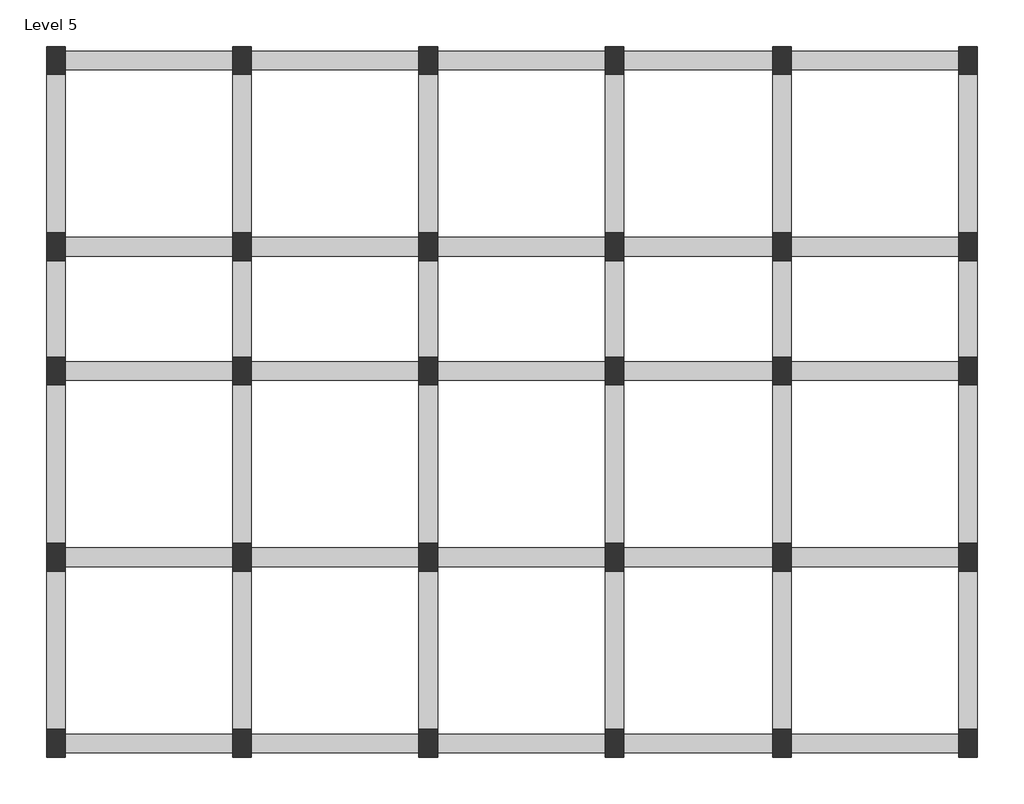
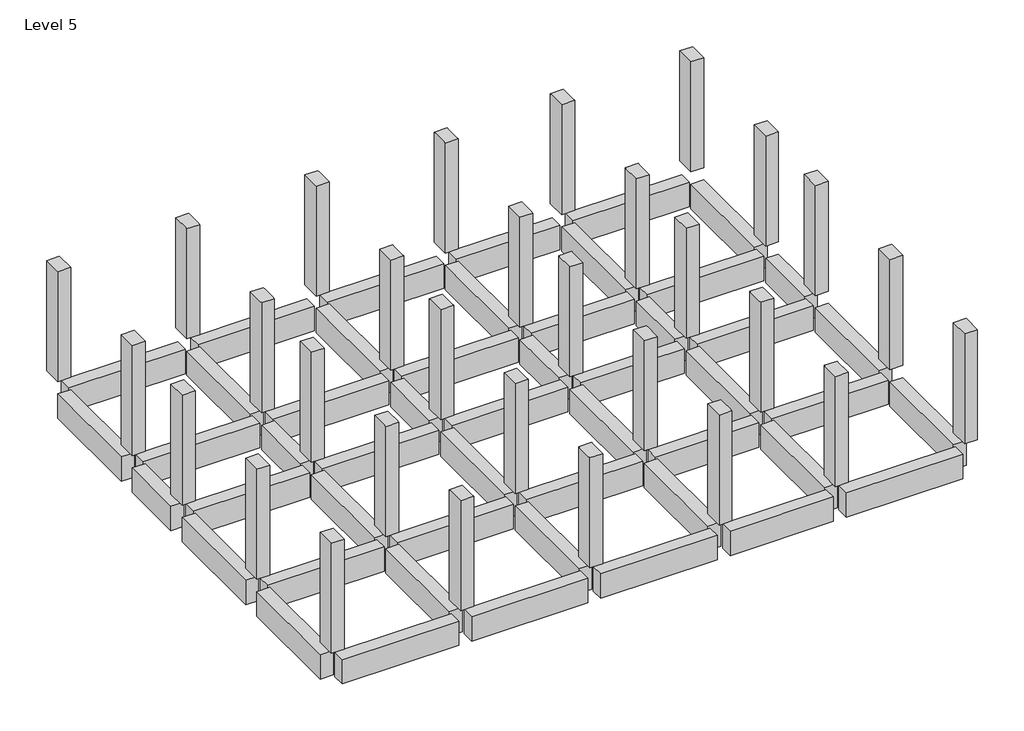
# One storey: 30 columns, 11 beams.
"""IFC4 building model written with IfcOpenShell, lengths in millimetres."""

from ifc_helpers import new_model, si_unit, frame, origin, place, context, project, spatial, polyline, outline, extrude, faceted_brep, element, save

model = new_model("IFC4")

# Units and contexts
model_context = context("Model", 3, world=origin())
ifc_project = project(units=[si_unit("LENGTHUNIT", "METRE", prefix="MILLI")], contexts=[model_context])

# Site, building, storey
site = spatial("IfcSite", under=ifc_project)
building = spatial("IfcBuilding", under=site)
storey = spatial("IfcBuildingStorey", under=building, Name="Level 5", Elevation=12192.0)

# Beams
placement = place(None, origin())
element("IfcBeam", 1, ObjectType="Concrete-Rectangular Beam : 12 x 24", at=placement, inside=storey, context=model_context, shape_type="SweptSolid", body=[
    extrude(outline(polyline([(2607.7603583, 7596.6647757), (2607.7603583, 7291.8647757), (-135.4396417, 7291.8647757), (-135.4396417, 7596.6647757), (2607.7603583, 7596.6647757)])), frame((0.0, 0.0, 11277.6), z_axis=(0.0, 0.0, 1.0), x_axis=(1.0, 0.0, 0.0)), (0.0, 0.0, 1.0), 609.6),
    extrude(outline(polyline([(-12022.6396417, 7291.8647757), (-12022.6396417, 7596.6647757), (-9279.4396417, 7596.6647757), (-9279.4396417, 7291.8647757), (-12022.6396417, 7291.8647757)])), frame((0.0, 0.0, 11277.6), z_axis=(0.0, 0.0, 1.0), x_axis=(1.0, 0.0, 0.0)), (0.0, 0.0, 1.0), 609.6),
    extrude(outline(polyline([(-8974.6396417, 7291.8647757), (-8974.6396417, 7596.6647757), (-6231.4396417, 7596.6647757), (-6231.4396417, 7291.8647757), (-8974.6396417, 7291.8647757)])), frame((0.0, 0.0, 11277.6), z_axis=(0.0, 0.0, 1.0), x_axis=(1.0, 0.0, 0.0)), (0.0, 0.0, 1.0), 609.6),
    extrude(outline(polyline([(-5926.6396417, 7291.8647757), (-5926.6396417, 7596.6647757), (-3183.4396417, 7596.6647757), (-3183.4396417, 7291.8647757), (-5926.6396417, 7291.8647757)])), frame((0.0, 0.0, 11277.6), z_axis=(0.0, 0.0, 1.0), x_axis=(1.0, 0.0, 0.0)), (0.0, 0.0, 1.0), 609.6),
    extrude(outline(polyline([(-2878.6396417, 7291.8647757), (-2878.6396417, 7596.6647757), (-440.2396417, 7596.6647757), (-440.2396417, 7291.8647757), (-2878.6396417, 7291.8647757)])), frame((0.0, 0.0, 11277.6), z_axis=(0.0, 0.0, 1.0), x_axis=(1.0, 0.0, 0.0)), (0.0, 0.0, 1.0), 609.6),
])
element("IfcBeam", 2, ObjectType="Concrete-Rectangular Beam : 12 x 24", at=placement, inside=storey, context=model_context, shape_type="SweptSolid", body=[
    extrude(outline(polyline([(2607.7603583, 10644.6647757), (2607.7603583, 10339.8647757), (-135.4396417, 10339.8647757), (-135.4396417, 10644.6647757), (2607.7603583, 10644.6647757)])), frame((0.0, 0.0, 11277.6), z_axis=(0.0, 0.0, 1.0), x_axis=(1.0, 0.0, 0.0)), (0.0, 0.0, 1.0), 609.6),
    extrude(outline(polyline([(-12022.6396417, 10339.8647757), (-12022.6396417, 10644.6647757), (-9279.4396417, 10644.6647757), (-9279.4396417, 10339.8647757), (-12022.6396417, 10339.8647757)])), frame((0.0, 0.0, 11277.6), z_axis=(0.0, 0.0, 1.0), x_axis=(1.0, 0.0, 0.0)), (0.0, 0.0, 1.0), 609.6),
    extrude(outline(polyline([(-8974.6396417, 10339.8647757), (-8974.6396417, 10644.6647757), (-6231.4396417, 10644.6647757), (-6231.4396417, 10339.8647757), (-8974.6396417, 10339.8647757)])), frame((0.0, 0.0, 11277.6), z_axis=(0.0, 0.0, 1.0), x_axis=(1.0, 0.0, 0.0)), (0.0, 0.0, 1.0), 609.6),
    extrude(outline(polyline([(-5926.6396417, 10339.8647757), (-5926.6396417, 10644.6647757), (-3183.4396417, 10644.6647757), (-3183.4396417, 10339.8647757), (-5926.6396417, 10339.8647757)])), frame((0.0, 0.0, 11277.6), z_axis=(0.0, 0.0, 1.0), x_axis=(1.0, 0.0, 0.0)), (0.0, 0.0, 1.0), 609.6),
    extrude(outline(polyline([(-2878.6396417, 10339.8647757), (-2878.6396417, 10644.6647757), (-440.2396417, 10644.6647757), (-440.2396417, 10339.8647757), (-2878.6396417, 10339.8647757)])), frame((0.0, 0.0, 11277.6), z_axis=(0.0, 0.0, 1.0), x_axis=(1.0, 0.0, 0.0)), (0.0, 0.0, 1.0), 609.6),
])
element("IfcBeam", 3, ObjectType="Concrete-Rectangular Beam : 12 x 24", at=placement, inside=storey, context=model_context, shape_type="SweptSolid", body=[
    extrude(outline(polyline([(2607.7603583, 13692.6647757), (2607.7603583, 13387.8647757), (-135.4396417, 13387.8647757), (-135.4396417, 13692.6647757), (2607.7603583, 13692.6647757)])), frame((0.0, 0.0, 11277.6), z_axis=(0.0, 0.0, 1.0), x_axis=(1.0, 0.0, 0.0)), (0.0, 0.0, 1.0), 609.6),
    extrude(outline(polyline([(-12022.6396417, 13387.8647757), (-12022.6396417, 13692.6647757), (-9279.4396417, 13692.6647757), (-9279.4396417, 13387.8647757), (-12022.6396417, 13387.8647757)])), frame((0.0, 0.0, 11277.6), z_axis=(0.0, 0.0, 1.0), x_axis=(1.0, 0.0, 0.0)), (0.0, 0.0, 1.0), 609.6),
    extrude(outline(polyline([(-8974.6396417, 13387.8647757), (-8974.6396417, 13692.6647757), (-6231.4396417, 13692.6647757), (-6231.4396417, 13387.8647757), (-8974.6396417, 13387.8647757)])), frame((0.0, 0.0, 11277.6), z_axis=(0.0, 0.0, 1.0), x_axis=(1.0, 0.0, 0.0)), (0.0, 0.0, 1.0), 609.6),
    extrude(outline(polyline([(-5926.6396417, 13387.8647757), (-5926.6396417, 13692.6647757), (-3183.4396417, 13692.6647757), (-3183.4396417, 13387.8647757), (-5926.6396417, 13387.8647757)])), frame((0.0, 0.0, 11277.6), z_axis=(0.0, 0.0, 1.0), x_axis=(1.0, 0.0, 0.0)), (0.0, 0.0, 1.0), 609.6),
    extrude(outline(polyline([(-2878.6396417, 13387.8647757), (-2878.6396417, 13692.6647757), (-440.2396417, 13692.6647757), (-440.2396417, 13387.8647757), (-2878.6396417, 13387.8647757)])), frame((0.0, 0.0, 11277.6), z_axis=(0.0, 0.0, 1.0), x_axis=(1.0, 0.0, 0.0)), (0.0, 0.0, 1.0), 609.6),
])
element("IfcBeam", 4, ObjectType="Concrete-Rectangular Beam : 12 x 24", at=placement, inside=storey, context=model_context, shape_type="SweptSolid", body=[
    extrude(outline(polyline([(2607.7603583, 15727.9119241), (2607.7603583, 15423.1119241), (-135.4396417, 15423.1119241), (-135.4396417, 15727.9119241), (2607.7603583, 15727.9119241)])), frame((0.0, 0.0, 11277.6), z_axis=(0.0, 0.0, 1.0), x_axis=(1.0, 0.0, 0.0)), (0.0, 0.0, 1.0), 609.6),
    extrude(outline(polyline([(-12022.6396417, 15423.1119241), (-12022.6396417, 15727.9119241), (-9279.4396417, 15727.9119241), (-9279.4396417, 15423.1119241), (-12022.6396417, 15423.1119241)])), frame((0.0, 0.0, 11277.6), z_axis=(0.0, 0.0, 1.0), x_axis=(1.0, 0.0, 0.0)), (0.0, 0.0, 1.0), 609.6),
    extrude(outline(polyline([(-8974.6396417, 15423.1119241), (-8974.6396417, 15727.9119241), (-6231.4396417, 15727.9119241), (-6231.4396417, 15423.1119241), (-8974.6396417, 15423.1119241)])), frame((0.0, 0.0, 11277.6), z_axis=(0.0, 0.0, 1.0), x_axis=(1.0, 0.0, 0.0)), (0.0, 0.0, 1.0), 609.6),
    extrude(outline(polyline([(-5926.6396417, 15423.1119241), (-5926.6396417, 15727.9119241), (-3183.4396417, 15727.9119241), (-3183.4396417, 15423.1119241), (-5926.6396417, 15423.1119241)])), frame((0.0, 0.0, 11277.6), z_axis=(0.0, 0.0, 1.0), x_axis=(1.0, 0.0, 0.0)), (0.0, 0.0, 1.0), 609.6),
    extrude(outline(polyline([(-2878.6396417, 15423.1119241), (-2878.6396417, 15727.9119241), (-440.2396417, 15727.9119241), (-440.2396417, 15423.1119241), (-2878.6396417, 15423.1119241)])), frame((0.0, 0.0, 11277.6), z_axis=(0.0, 0.0, 1.0), x_axis=(1.0, 0.0, 0.0)), (0.0, 0.0, 1.0), 609.6),
])
element("IfcBeam", 5, ObjectType="Concrete-Rectangular Beam : 12 x 24", at=placement, inside=storey, context=model_context, shape_type="SweptSolid", body=[
    extrude(outline(polyline([(2607.7603583, 18775.9119241), (2607.7603583, 18471.1119241), (-135.4396417, 18471.1119241), (-135.4396417, 18775.9119241), (2607.7603583, 18775.9119241)])), frame((0.0, 0.0, 11277.6), z_axis=(0.0, 0.0, 1.0), x_axis=(1.0, 0.0, 0.0)), (0.0, 0.0, 1.0), 609.6),
    extrude(outline(polyline([(-12022.6396417, 18471.1119241), (-12022.6396417, 18775.9119241), (-9279.4396417, 18775.9119241), (-9279.4396417, 18471.1119241), (-12022.6396417, 18471.1119241)])), frame((0.0, 0.0, 11277.6), z_axis=(0.0, 0.0, 1.0), x_axis=(1.0, 0.0, 0.0)), (0.0, 0.0, 1.0), 609.6),
    extrude(outline(polyline([(-8974.6396417, 18471.1119241), (-8974.6396417, 18775.9119241), (-6231.4396417, 18775.9119241), (-6231.4396417, 18471.1119241), (-8974.6396417, 18471.1119241)])), frame((0.0, 0.0, 11277.6), z_axis=(0.0, 0.0, 1.0), x_axis=(1.0, 0.0, 0.0)), (0.0, 0.0, 1.0), 609.6),
    extrude(outline(polyline([(-5926.6396417, 18471.1119241), (-5926.6396417, 18775.9119241), (-3183.4396417, 18775.9119241), (-3183.4396417, 18471.1119241), (-5926.6396417, 18471.1119241)])), frame((0.0, 0.0, 11277.6), z_axis=(0.0, 0.0, 1.0), x_axis=(1.0, 0.0, 0.0)), (0.0, 0.0, 1.0), 609.6),
    extrude(outline(polyline([(-2878.6396417, 18471.1119241), (-2878.6396417, 18775.9119241), (-440.2396417, 18775.9119241), (-440.2396417, 18471.1119241), (-2878.6396417, 18471.1119241)])), frame((0.0, 0.0, 11277.6), z_axis=(0.0, 0.0, 1.0), x_axis=(1.0, 0.0, 0.0)), (0.0, 0.0, 1.0), 609.6),
])
element("IfcBeam", 6, ObjectType="Concrete-Rectangular Beam : 12 x 24", at=placement, inside=storey, context=model_context, shape_type="SweptSolid", body=[
    extrude(outline(polyline([(-12022.6396417, 7672.8647757), (-12327.4396417, 7672.8647757), (-12327.4396417, 10263.6647757), (-12022.6396417, 10263.6647757), (-12022.6396417, 7672.8647757)])), frame((0.0, 0.0, 11277.6), z_axis=(0.0, 0.0, 1.0), x_axis=(1.0, 0.0, 0.0)), (0.0, 0.0, 1.0), 609.6),
    extrude(outline(polyline([(-12327.4396417, 18394.9119241), (-12022.6396417, 18394.9119241), (-12022.6396417, 15804.1119241), (-12327.4396417, 15804.1119241), (-12327.4396417, 18394.9119241)])), frame((0.0, 0.0, 11277.6), z_axis=(0.0, 0.0, 1.0), x_axis=(1.0, 0.0, 0.0)), (0.0, 0.0, 1.0), 609.6),
    extrude(outline(polyline([(-12022.6396417, 10720.8647757), (-12327.4396417, 10720.8647757), (-12327.4396417, 13311.6647757), (-12022.6396417, 13311.6647757), (-12022.6396417, 10720.8647757)])), frame((0.0, 0.0, 11277.6), z_axis=(0.0, 0.0, 1.0), x_axis=(1.0, 0.0, 0.0)), (0.0, 0.0, 1.0), 609.6),
    extrude(outline(polyline([(-12022.6396417, 13768.8647757), (-12327.4396417, 13768.8647757), (-12327.4396417, 15346.9119241), (-12022.6396417, 15346.9119241), (-12022.6396417, 13768.8647757)])), frame((0.0, 0.0, 11277.6), z_axis=(0.0, 0.0, 1.0), x_axis=(1.0, 0.0, 0.0)), (0.0, 0.0, 1.0), 609.6),
])
element("IfcBeam", 7, ObjectType="Concrete-Rectangular Beam : 12 x 24", at=placement, inside=storey, context=model_context, shape_type="SweptSolid", body=[
    extrude(outline(polyline([(-8974.6396417, 7672.8647757), (-9279.4396417, 7672.8647757), (-9279.4396417, 10263.6647757), (-8974.6396417, 10263.6647757), (-8974.6396417, 7672.8647757)])), frame((0.0, 0.0, 11277.6), z_axis=(0.0, 0.0, 1.0), x_axis=(1.0, 0.0, 0.0)), (0.0, 0.0, 1.0), 609.6),
    extrude(outline(polyline([(-9279.4396417, 18394.9119241), (-8974.6396417, 18394.9119241), (-8974.6396417, 15804.1119241), (-9279.4396417, 15804.1119241), (-9279.4396417, 18394.9119241)])), frame((0.0, 0.0, 11277.6), z_axis=(0.0, 0.0, 1.0), x_axis=(1.0, 0.0, 0.0)), (0.0, 0.0, 1.0), 609.6),
    extrude(outline(polyline([(-8974.6396417, 10720.8647757), (-9279.4396417, 10720.8647757), (-9279.4396417, 13311.6647757), (-8974.6396417, 13311.6647757), (-8974.6396417, 10720.8647757)])), frame((0.0, 0.0, 11277.6), z_axis=(0.0, 0.0, 1.0), x_axis=(1.0, 0.0, 0.0)), (0.0, 0.0, 1.0), 609.6),
    extrude(outline(polyline([(-8974.6396417, 13768.8647757), (-9279.4396417, 13768.8647757), (-9279.4396417, 15346.9119241), (-8974.6396417, 15346.9119241), (-8974.6396417, 13768.8647757)])), frame((0.0, 0.0, 11277.6), z_axis=(0.0, 0.0, 1.0), x_axis=(1.0, 0.0, 0.0)), (0.0, 0.0, 1.0), 609.6),
])
element("IfcBeam", 8, ObjectType="Concrete-Rectangular Beam : 12 x 24", at=placement, inside=storey, context=model_context, shape_type="SweptSolid", body=[
    extrude(outline(polyline([(-5926.6396417, 7672.8647757), (-6231.4396417, 7672.8647757), (-6231.4396417, 10263.6647757), (-5926.6396417, 10263.6647757), (-5926.6396417, 7672.8647757)])), frame((0.0, 0.0, 11277.6), z_axis=(0.0, 0.0, 1.0), x_axis=(1.0, 0.0, 0.0)), (0.0, 0.0, 1.0), 609.6),
    extrude(outline(polyline([(-6231.4396417, 18394.9119241), (-5926.6396417, 18394.9119241), (-5926.6396417, 15804.1119241), (-6231.4396417, 15804.1119241), (-6231.4396417, 18394.9119241)])), frame((0.0, 0.0, 11277.6), z_axis=(0.0, 0.0, 1.0), x_axis=(1.0, 0.0, 0.0)), (0.0, 0.0, 1.0), 609.6),
    extrude(outline(polyline([(-5926.6396417, 10720.8647757), (-6231.4396417, 10720.8647757), (-6231.4396417, 13311.6647757), (-5926.6396417, 13311.6647757), (-5926.6396417, 10720.8647757)])), frame((0.0, 0.0, 11277.6), z_axis=(0.0, 0.0, 1.0), x_axis=(1.0, 0.0, 0.0)), (0.0, 0.0, 1.0), 609.6),
    extrude(outline(polyline([(-5926.6396417, 13768.8647757), (-6231.4396417, 13768.8647757), (-6231.4396417, 15346.9119241), (-5926.6396417, 15346.9119241), (-5926.6396417, 13768.8647757)])), frame((0.0, 0.0, 11277.6), z_axis=(0.0, 0.0, 1.0), x_axis=(1.0, 0.0, 0.0)), (0.0, 0.0, 1.0), 609.6),
])
element("IfcBeam", 9, ObjectType="Concrete-Rectangular Beam : 12 x 24", at=placement, inside=storey, context=model_context, shape_type="SweptSolid", body=[
    extrude(outline(polyline([(-2878.6396417, 7672.8647757), (-3183.4396417, 7672.8647757), (-3183.4396417, 10263.6647757), (-2878.6396417, 10263.6647757), (-2878.6396417, 7672.8647757)])), frame((0.0, 0.0, 11277.6), z_axis=(0.0, 0.0, 1.0), x_axis=(1.0, 0.0, 0.0)), (0.0, 0.0, 1.0), 609.6),
    extrude(outline(polyline([(-3183.4396417, 18394.9119241), (-2878.6396417, 18394.9119241), (-2878.6396417, 15804.1119241), (-3183.4396417, 15804.1119241), (-3183.4396417, 18394.9119241)])), frame((0.0, 0.0, 11277.6), z_axis=(0.0, 0.0, 1.0), x_axis=(1.0, 0.0, 0.0)), (0.0, 0.0, 1.0), 609.6),
    extrude(outline(polyline([(-2878.6396417, 10720.8647757), (-3183.4396417, 10720.8647757), (-3183.4396417, 13311.6647757), (-2878.6396417, 13311.6647757), (-2878.6396417, 10720.8647757)])), frame((0.0, 0.0, 11277.6), z_axis=(0.0, 0.0, 1.0), x_axis=(1.0, 0.0, 0.0)), (0.0, 0.0, 1.0), 609.6),
    extrude(outline(polyline([(-2878.6396417, 13768.8647757), (-3183.4396417, 13768.8647757), (-3183.4396417, 15346.9119241), (-2878.6396417, 15346.9119241), (-2878.6396417, 13768.8647757)])), frame((0.0, 0.0, 11277.6), z_axis=(0.0, 0.0, 1.0), x_axis=(1.0, 0.0, 0.0)), (0.0, 0.0, 1.0), 609.6),
])
element("IfcBeam", 10, ObjectType="Concrete-Rectangular Beam : 12 x 24", at=placement, inside=storey, context=model_context, shape_type="SweptSolid", body=[
    extrude(outline(polyline([(-135.4396417, 7672.8647757), (-440.2396417, 7672.8647757), (-440.2396417, 10263.6647757), (-135.4396417, 10263.6647757), (-135.4396417, 7672.8647757)])), frame((0.0, 0.0, 11277.6), z_axis=(0.0, 0.0, 1.0), x_axis=(1.0, 0.0, 0.0)), (0.0, 0.0, 1.0), 609.6),
    extrude(outline(polyline([(-440.2396417, 18394.9119241), (-135.4396417, 18394.9119241), (-135.4396417, 15804.1119241), (-440.2396417, 15804.1119241), (-440.2396417, 18394.9119241)])), frame((0.0, 0.0, 11277.6), z_axis=(0.0, 0.0, 1.0), x_axis=(1.0, 0.0, 0.0)), (0.0, 0.0, 1.0), 609.6),
    extrude(outline(polyline([(-135.4396417, 10720.8647757), (-440.2396417, 10720.8647757), (-440.2396417, 13311.6647757), (-135.4396417, 13311.6647757), (-135.4396417, 10720.8647757)])), frame((0.0, 0.0, 11277.6), z_axis=(0.0, 0.0, 1.0), x_axis=(1.0, 0.0, 0.0)), (0.0, 0.0, 1.0), 609.6),
    extrude(outline(polyline([(-135.4396417, 13768.8647757), (-440.2396417, 13768.8647757), (-440.2396417, 15346.9119241), (-135.4396417, 15346.9119241), (-135.4396417, 13768.8647757)])), frame((0.0, 0.0, 11277.6), z_axis=(0.0, 0.0, 1.0), x_axis=(1.0, 0.0, 0.0)), (0.0, 0.0, 1.0), 609.6),
])
element("IfcBeam", 11, ObjectType="Concrete-Rectangular Beam : 12 x 24", at=placement, inside=storey, context=model_context, shape_type="SweptSolid", body=[
    extrude(outline(polyline([(2912.5603583, 7672.8647757), (2607.7603583, 7672.8647757), (2607.7603583, 10263.6647757), (2912.5603583, 10263.6647757), (2912.5603583, 7672.8647757)])), frame((0.0, 0.0, 11277.6), z_axis=(0.0, 0.0, 1.0), x_axis=(1.0, 0.0, 0.0)), (0.0, 0.0, 1.0), 609.6),
    extrude(outline(polyline([(2607.7603583, 18394.9119241), (2912.5603583, 18394.9119241), (2912.5603583, 15804.1119241), (2607.7603583, 15804.1119241), (2607.7603583, 18394.9119241)])), frame((0.0, 0.0, 11277.6), z_axis=(0.0, 0.0, 1.0), x_axis=(1.0, 0.0, 0.0)), (0.0, 0.0, 1.0), 609.6),
    extrude(outline(polyline([(2912.5603583, 10720.8647757), (2607.7603583, 10720.8647757), (2607.7603583, 13311.6647757), (2912.5603583, 13311.6647757), (2912.5603583, 10720.8647757)])), frame((0.0, 0.0, 11277.6), z_axis=(0.0, 0.0, 1.0), x_axis=(1.0, 0.0, 0.0)), (0.0, 0.0, 1.0), 609.6),
    extrude(outline(polyline([(2912.5603583, 13768.8647757), (2607.7603583, 13768.8647757), (2607.7603583, 15346.9119241), (2912.5603583, 15346.9119241), (2912.5603583, 13768.8647757)])), frame((0.0, 0.0, 11277.6), z_axis=(0.0, 0.0, 1.0), x_axis=(1.0, 0.0, 0.0)), (0.0, 0.0, 1.0), 609.6),
])

# Columns
element("IfcColumn", 12, ObjectType="Concrete-Rectangular-Column : c1", at=placement, inside=storey, context=model_context, shape_type="SweptSolid", body=[
    extrude(outline(polyline([(-12327.4396417, 7215.6647757), (-12327.4396417, 7672.8647757), (-12022.6396417, 7672.8647757), (-12022.6396417, 7215.6647757), (-12327.4396417, 7215.6647757)])), frame((0.0, 0.0, 12192.0), z_axis=(0.0, 0.0, 1.0), x_axis=(1.0, 0.0, 0.0)), (0.0, 0.0, 1.0), 2743.2),
])
element("IfcColumn", 13, ObjectType="Concrete-Rectangular-Column : c1", at=placement, inside=storey, context=model_context, shape_type="Brep", body=[
    faceted_brep([(-9279.4396417, 7215.6647757, 12192.0), (-9279.4396417, 7672.8647757, 12192.0), (-8974.6396417, 7672.8647757, 12192.0), (-8974.6396417, 7215.6647757, 12192.0), (-9279.4396417, 7215.6647757, 14935.2), (-9279.4396417, 7291.8647757, 14935.2), (-9279.4396417, 7596.6647757, 14935.2), (-9279.4396417, 7672.8647757, 14935.2), (-8974.6396417, 7672.8647757, 14935.2), (-8974.6396417, 7596.6647757, 14935.2), (-8974.6396417, 7291.8647757, 14935.2), (-8974.6396417, 7215.6647757, 14935.2)], [[[0, 1, 2, 3]], [[4, 5, 6, 7, 1, 0]], [[7, 8, 2, 1]], [[8, 9, 10, 11, 3, 2]], [[11, 4, 0, 3]], [[4, 11, 10, 9, 8, 7, 6, 5]]]),
])
element("IfcColumn", 14, ObjectType="Concrete-Rectangular-Column : c1", at=placement, inside=storey, context=model_context, shape_type="Brep", body=[
    faceted_brep([(-6231.4396417, 7215.6647757, 12192.0), (-6231.4396417, 7672.8647757, 12192.0), (-5926.6396417, 7672.8647757, 12192.0), (-5926.6396417, 7215.6647757, 12192.0), (-6231.4396417, 7215.6647757, 14935.2), (-6231.4396417, 7291.8647757, 14935.2), (-6231.4396417, 7596.6647757, 14935.2), (-6231.4396417, 7672.8647757, 14935.2), (-5926.6396417, 7672.8647757, 14935.2), (-5926.6396417, 7596.6647757, 14935.2), (-5926.6396417, 7291.8647757, 14935.2), (-5926.6396417, 7215.6647757, 14935.2)], [[[0, 1, 2, 3]], [[4, 5, 6, 7, 1, 0]], [[7, 8, 2, 1]], [[8, 9, 10, 11, 3, 2]], [[11, 4, 0, 3]], [[4, 11, 10, 9, 8, 7, 6, 5]]]),
])
element("IfcColumn", 15, ObjectType="Concrete-Rectangular-Column : c1", at=placement, inside=storey, context=model_context, shape_type="Brep", body=[
    faceted_brep([(-3183.4396417, 7215.6647757, 12192.0), (-3183.4396417, 7672.8647757, 12192.0), (-2878.6396417, 7672.8647757, 12192.0), (-2878.6396417, 7215.6647757, 12192.0), (-3183.4396417, 7215.6647757, 14935.2), (-3183.4396417, 7291.8647757, 14935.2), (-3183.4396417, 7596.6647757, 14935.2), (-3183.4396417, 7672.8647757, 14935.2), (-2878.6396417, 7672.8647757, 14935.2), (-2878.6396417, 7596.6647757, 14935.2), (-2878.6396417, 7291.8647757, 14935.2), (-2878.6396417, 7215.6647757, 14935.2)], [[[0, 1, 2, 3]], [[4, 5, 6, 7, 1, 0]], [[7, 8, 2, 1]], [[8, 9, 10, 11, 3, 2]], [[11, 4, 0, 3]], [[4, 11, 10, 9, 8, 7, 6, 5]]]),
])
element("IfcColumn", 16, ObjectType="Concrete-Rectangular-Column : c1", at=placement, inside=storey, context=model_context, shape_type="Brep", body=[
    faceted_brep([(-440.2396417, 7215.6647757, 12192.0), (-440.2396417, 7672.8647757, 12192.0), (-135.4396417, 7672.8647757, 12192.0), (-135.4396417, 7215.6647757, 12192.0), (-440.2396417, 7215.6647757, 14935.2), (-440.2396417, 7291.8647757, 14935.2), (-440.2396417, 7596.6647757, 14935.2), (-440.2396417, 7672.8647757, 14935.2), (-135.4396417, 7672.8647757, 14935.2), (-135.4396417, 7596.6647757, 14935.2), (-135.4396417, 7291.8647757, 14935.2), (-135.4396417, 7215.6647757, 14935.2)], [[[0, 1, 2, 3]], [[4, 5, 6, 7, 1, 0]], [[7, 8, 2, 1]], [[8, 9, 10, 11, 3, 2]], [[11, 4, 0, 3]], [[4, 11, 10, 9, 8, 7, 6, 5]]]),
])
element("IfcColumn", 17, ObjectType="Concrete-Rectangular-Column : c1", at=placement, inside=storey, context=model_context, shape_type="SweptSolid", body=[
    extrude(outline(polyline([(2607.7603583, 7215.6647757), (2607.7603583, 7672.8647757), (2912.5603583, 7672.8647757), (2912.5603583, 7215.6647757), (2607.7603583, 7215.6647757)])), frame((0.0, 0.0, 12192.0), z_axis=(0.0, 0.0, 1.0), x_axis=(1.0, 0.0, 0.0)), (0.0, 0.0, 1.0), 2743.2),
])
element("IfcColumn", 18, ObjectType="Concrete-Rectangular-Column : c1", at=placement, inside=storey, context=model_context, shape_type="Brep", body=[
    faceted_brep([(-12327.4396417, 10263.6647757, 12192.0), (-12327.4396417, 10720.8647757, 12192.0), (-12022.6396417, 10720.8647757, 12192.0), (-12022.6396417, 10263.6647757, 12192.0), (-12327.4396417, 10263.6647757, 14935.2), (-12327.4396417, 10720.8647757, 14935.2), (-12327.4396417, 10720.8647757, 14325.6), (-12327.4396417, 10263.6647757, 14325.6), (-12022.6396417, 10720.8647757, 14935.2), (-12022.6396417, 10720.8647757, 14325.6), (-12022.6396417, 10263.6647757, 14935.2), (-12022.6396417, 10263.6647757, 14325.6)], [[[0, 1, 2, 3]], [[4, 5, 6, 1, 0, 7]], [[5, 8, 9, 2, 1, 6]], [[8, 10, 11, 3, 2, 9]], [[10, 4, 7, 0, 3, 11]], [[4, 10, 8, 5]]]),
])
element("IfcColumn", 19, ObjectType="Concrete-Rectangular-Column : c1", at=placement, inside=storey, context=model_context, shape_type="Brep", body=[
    faceted_brep([(-9279.4396417, 10263.6647757, 12192.0), (-9279.4396417, 10720.8647757, 12192.0), (-8974.6396417, 10720.8647757, 12192.0), (-8974.6396417, 10263.6647757, 12192.0), (-9279.4396417, 10263.6647757, 14935.2), (-9279.4396417, 10339.8647757, 14935.2), (-9279.4396417, 10644.6647757, 14935.2), (-9279.4396417, 10720.8647757, 14935.2), (-9279.4396417, 10720.8647757, 14325.6), (-9279.4396417, 10263.6647757, 14325.6), (-8974.6396417, 10720.8647757, 14935.2), (-8974.6396417, 10720.8647757, 14325.6), (-8974.6396417, 10644.6647757, 14935.2), (-8974.6396417, 10339.8647757, 14935.2), (-8974.6396417, 10263.6647757, 14935.2), (-8974.6396417, 10263.6647757, 14325.6)], [[[0, 1, 2, 3]], [[4, 5, 6, 7, 8, 1, 0, 9]], [[7, 10, 11, 2, 1, 8]], [[10, 12, 13, 14, 15, 3, 2, 11]], [[14, 4, 9, 0, 3, 15]], [[4, 14, 13, 12, 10, 7, 6, 5]]]),
])
element("IfcColumn", 20, ObjectType="Concrete-Rectangular-Column : c1", at=placement, inside=storey, context=model_context, shape_type="Brep", body=[
    faceted_brep([(-6231.4396417, 10263.6647757, 12192.0), (-6231.4396417, 10720.8647757, 12192.0), (-5926.6396417, 10720.8647757, 12192.0), (-5926.6396417, 10263.6647757, 12192.0), (-6231.4396417, 10263.6647757, 14935.2), (-6231.4396417, 10339.8647757, 14935.2), (-6231.4396417, 10644.6647757, 14935.2), (-6231.4396417, 10720.8647757, 14935.2), (-6231.4396417, 10720.8647757, 14325.6), (-6231.4396417, 10263.6647757, 14325.6), (-5926.6396417, 10720.8647757, 14935.2), (-5926.6396417, 10720.8647757, 14325.6), (-5926.6396417, 10644.6647757, 14935.2), (-5926.6396417, 10339.8647757, 14935.2), (-5926.6396417, 10263.6647757, 14935.2), (-5926.6396417, 10263.6647757, 14325.6)], [[[0, 1, 2, 3]], [[4, 5, 6, 7, 8, 1, 0, 9]], [[7, 10, 11, 2, 1, 8]], [[10, 12, 13, 14, 15, 3, 2, 11]], [[14, 4, 9, 0, 3, 15]], [[4, 14, 13, 12, 10, 7, 6, 5]]]),
])
element("IfcColumn", 21, ObjectType="Concrete-Rectangular-Column : c1", at=placement, inside=storey, context=model_context, shape_type="Brep", body=[
    faceted_brep([(-3183.4396417, 10263.6647757, 12192.0), (-3183.4396417, 10720.8647757, 12192.0), (-2878.6396417, 10720.8647757, 12192.0), (-2878.6396417, 10263.6647757, 12192.0), (-3183.4396417, 10263.6647757, 14935.2), (-3183.4396417, 10339.8647757, 14935.2), (-3183.4396417, 10644.6647757, 14935.2), (-3183.4396417, 10720.8647757, 14935.2), (-3183.4396417, 10720.8647757, 14325.6), (-3183.4396417, 10263.6647757, 14325.6), (-2878.6396417, 10720.8647757, 14935.2), (-2878.6396417, 10720.8647757, 14325.6), (-2878.6396417, 10644.6647757, 14935.2), (-2878.6396417, 10339.8647757, 14935.2), (-2878.6396417, 10263.6647757, 14935.2), (-2878.6396417, 10263.6647757, 14325.6)], [[[0, 1, 2, 3]], [[4, 5, 6, 7, 8, 1, 0, 9]], [[7, 10, 11, 2, 1, 8]], [[10, 12, 13, 14, 15, 3, 2, 11]], [[14, 4, 9, 0, 3, 15]], [[4, 14, 13, 12, 10, 7, 6, 5]]]),
])
element("IfcColumn", 22, ObjectType="Concrete-Rectangular-Column : c1", at=placement, inside=storey, context=model_context, shape_type="Brep", body=[
    faceted_brep([(-440.2396417, 10263.6647757, 12192.0), (-440.2396417, 10720.8647757, 12192.0), (-135.4396417, 10720.8647757, 12192.0), (-135.4396417, 10263.6647757, 12192.0), (-440.2396417, 10263.6647757, 14935.2), (-440.2396417, 10339.8647757, 14935.2), (-440.2396417, 10644.6647757, 14935.2), (-440.2396417, 10720.8647757, 14935.2), (-440.2396417, 10720.8647757, 14325.6), (-440.2396417, 10263.6647757, 14325.6), (-135.4396417, 10720.8647757, 14935.2), (-135.4396417, 10720.8647757, 14325.6), (-135.4396417, 10644.6647757, 14935.2), (-135.4396417, 10339.8647757, 14935.2), (-135.4396417, 10263.6647757, 14935.2), (-135.4396417, 10263.6647757, 14325.6)], [[[0, 1, 2, 3]], [[4, 5, 6, 7, 8, 1, 0, 9]], [[7, 10, 11, 2, 1, 8]], [[10, 12, 13, 14, 15, 3, 2, 11]], [[14, 4, 9, 0, 3, 15]], [[4, 14, 13, 12, 10, 7, 6, 5]]]),
])
element("IfcColumn", 23, ObjectType="Concrete-Rectangular-Column : c1", at=placement, inside=storey, context=model_context, shape_type="Brep", body=[
    faceted_brep([(2607.7603583, 10263.6647757, 12192.0), (2607.7603583, 10720.8647757, 12192.0), (2912.5603583, 10720.8647757, 12192.0), (2912.5603583, 10263.6647757, 12192.0), (2607.7603583, 10263.6647757, 14935.2), (2607.7603583, 10720.8647757, 14935.2), (2607.7603583, 10720.8647757, 14325.6), (2607.7603583, 10263.6647757, 14325.6), (2912.5603583, 10720.8647757, 14935.2), (2912.5603583, 10720.8647757, 14325.6), (2912.5603583, 10263.6647757, 14935.2), (2912.5603583, 10263.6647757, 14325.6)], [[[0, 1, 2, 3]], [[4, 5, 6, 1, 0, 7]], [[5, 8, 9, 2, 1, 6]], [[8, 10, 11, 3, 2, 9]], [[10, 4, 7, 0, 3, 11]], [[4, 10, 8, 5]]]),
])
element("IfcColumn", 24, ObjectType="Concrete-Rectangular-Column : c1", at=placement, inside=storey, context=model_context, shape_type="Brep", body=[
    faceted_brep([(-12327.4396417, 13311.6647757, 12192.0), (-12327.4396417, 13768.8647757, 12192.0), (-12022.6396417, 13768.8647757, 12192.0), (-12022.6396417, 13311.6647757, 12192.0), (-12327.4396417, 13311.6647757, 14935.2), (-12327.4396417, 13768.8647757, 14935.2), (-12327.4396417, 13768.8647757, 14325.6), (-12327.4396417, 13311.6647757, 14325.6), (-12022.6396417, 13768.8647757, 14935.2), (-12022.6396417, 13768.8647757, 14325.6), (-12022.6396417, 13311.6647757, 14935.2), (-12022.6396417, 13311.6647757, 14325.6)], [[[0, 1, 2, 3]], [[4, 5, 6, 1, 0, 7]], [[5, 8, 9, 2, 1, 6]], [[8, 10, 11, 3, 2, 9]], [[10, 4, 7, 0, 3, 11]], [[4, 10, 8, 5]]]),
])
element("IfcColumn", 25, ObjectType="Concrete-Rectangular-Column : c1", at=placement, inside=storey, context=model_context, shape_type="Brep", body=[
    faceted_brep([(-9279.4396417, 13311.6647757, 12192.0), (-9279.4396417, 13768.8647757, 12192.0), (-8974.6396417, 13768.8647757, 12192.0), (-8974.6396417, 13311.6647757, 12192.0), (-9279.4396417, 13311.6647757, 14935.2), (-9279.4396417, 13387.8647757, 14935.2), (-9279.4396417, 13692.6647757, 14935.2), (-9279.4396417, 13768.8647757, 14935.2), (-9279.4396417, 13768.8647757, 14325.6), (-9279.4396417, 13311.6647757, 14325.6), (-8974.6396417, 13768.8647757, 14935.2), (-8974.6396417, 13768.8647757, 14325.6), (-8974.6396417, 13692.6647757, 14935.2), (-8974.6396417, 13387.8647757, 14935.2), (-8974.6396417, 13311.6647757, 14935.2), (-8974.6396417, 13311.6647757, 14325.6)], [[[0, 1, 2, 3]], [[4, 5, 6, 7, 8, 1, 0, 9]], [[7, 10, 11, 2, 1, 8]], [[10, 12, 13, 14, 15, 3, 2, 11]], [[14, 4, 9, 0, 3, 15]], [[4, 14, 13, 12, 10, 7, 6, 5]]]),
])
element("IfcColumn", 26, ObjectType="Concrete-Rectangular-Column : c1", at=placement, inside=storey, context=model_context, shape_type="Brep", body=[
    faceted_brep([(-6231.4396417, 13311.6647757, 12192.0), (-6231.4396417, 13768.8647757, 12192.0), (-5926.6396417, 13768.8647757, 12192.0), (-5926.6396417, 13311.6647757, 12192.0), (-6231.4396417, 13311.6647757, 14935.2), (-6231.4396417, 13387.8647757, 14935.2), (-6231.4396417, 13692.6647757, 14935.2), (-6231.4396417, 13768.8647757, 14935.2), (-6231.4396417, 13768.8647757, 14325.6), (-6231.4396417, 13311.6647757, 14325.6), (-5926.6396417, 13768.8647757, 14935.2), (-5926.6396417, 13768.8647757, 14325.6), (-5926.6396417, 13692.6647757, 14935.2), (-5926.6396417, 13387.8647757, 14935.2), (-5926.6396417, 13311.6647757, 14935.2), (-5926.6396417, 13311.6647757, 14325.6)], [[[0, 1, 2, 3]], [[4, 5, 6, 7, 8, 1, 0, 9]], [[7, 10, 11, 2, 1, 8]], [[10, 12, 13, 14, 15, 3, 2, 11]], [[14, 4, 9, 0, 3, 15]], [[4, 14, 13, 12, 10, 7, 6, 5]]]),
])
element("IfcColumn", 27, ObjectType="Concrete-Rectangular-Column : c1", at=placement, inside=storey, context=model_context, shape_type="Brep", body=[
    faceted_brep([(-3183.4396417, 13311.6647757, 12192.0), (-3183.4396417, 13768.8647757, 12192.0), (-2878.6396417, 13768.8647757, 12192.0), (-2878.6396417, 13311.6647757, 12192.0), (-3183.4396417, 13311.6647757, 14935.2), (-3183.4396417, 13387.8647757, 14935.2), (-3183.4396417, 13692.6647757, 14935.2), (-3183.4396417, 13768.8647757, 14935.2), (-3183.4396417, 13768.8647757, 14325.6), (-3183.4396417, 13311.6647757, 14325.6), (-2878.6396417, 13768.8647757, 14935.2), (-2878.6396417, 13768.8647757, 14325.6), (-2878.6396417, 13692.6647757, 14935.2), (-2878.6396417, 13387.8647757, 14935.2), (-2878.6396417, 13311.6647757, 14935.2), (-2878.6396417, 13311.6647757, 14325.6)], [[[0, 1, 2, 3]], [[4, 5, 6, 7, 8, 1, 0, 9]], [[7, 10, 11, 2, 1, 8]], [[10, 12, 13, 14, 15, 3, 2, 11]], [[14, 4, 9, 0, 3, 15]], [[4, 14, 13, 12, 10, 7, 6, 5]]]),
])
element("IfcColumn", 28, ObjectType="Concrete-Rectangular-Column : c1", at=placement, inside=storey, context=model_context, shape_type="Brep", body=[
    faceted_brep([(-440.2396417, 13311.6647757, 12192.0), (-440.2396417, 13768.8647757, 12192.0), (-135.4396417, 13768.8647757, 12192.0), (-135.4396417, 13311.6647757, 12192.0), (-440.2396417, 13311.6647757, 14935.2), (-440.2396417, 13387.8647757, 14935.2), (-440.2396417, 13692.6647757, 14935.2), (-440.2396417, 13768.8647757, 14935.2), (-440.2396417, 13768.8647757, 14325.6), (-440.2396417, 13311.6647757, 14325.6), (-135.4396417, 13768.8647757, 14935.2), (-135.4396417, 13768.8647757, 14325.6), (-135.4396417, 13692.6647757, 14935.2), (-135.4396417, 13387.8647757, 14935.2), (-135.4396417, 13311.6647757, 14935.2), (-135.4396417, 13311.6647757, 14325.6)], [[[0, 1, 2, 3]], [[4, 5, 6, 7, 8, 1, 0, 9]], [[7, 10, 11, 2, 1, 8]], [[10, 12, 13, 14, 15, 3, 2, 11]], [[14, 4, 9, 0, 3, 15]], [[4, 14, 13, 12, 10, 7, 6, 5]]]),
])
element("IfcColumn", 29, ObjectType="Concrete-Rectangular-Column : c1", at=placement, inside=storey, context=model_context, shape_type="Brep", body=[
    faceted_brep([(2607.7603583, 13311.6647757, 12192.0), (2607.7603583, 13768.8647757, 12192.0), (2912.5603583, 13768.8647757, 12192.0), (2912.5603583, 13311.6647757, 12192.0), (2607.7603583, 13311.6647757, 14935.2), (2607.7603583, 13768.8647757, 14935.2), (2607.7603583, 13768.8647757, 14325.6), (2607.7603583, 13311.6647757, 14325.6), (2912.5603583, 13768.8647757, 14935.2), (2912.5603583, 13768.8647757, 14325.6), (2912.5603583, 13311.6647757, 14935.2), (2912.5603583, 13311.6647757, 14325.6)], [[[0, 1, 2, 3]], [[4, 5, 6, 1, 0, 7]], [[5, 8, 9, 2, 1, 6]], [[8, 10, 11, 3, 2, 9]], [[10, 4, 7, 0, 3, 11]], [[4, 10, 8, 5]]]),
])
element("IfcColumn", 30, ObjectType="Concrete-Rectangular-Column : c1", at=placement, inside=storey, context=model_context, shape_type="Brep", body=[
    faceted_brep([(-12327.4396417, 15346.9119241, 12192.0), (-12327.4396417, 15804.1119241, 12192.0), (-12022.6396417, 15804.1119241, 12192.0), (-12022.6396417, 15346.9119241, 12192.0), (-12327.4396417, 15346.9119241, 14935.2), (-12327.4396417, 15804.1119241, 14935.2), (-12327.4396417, 15804.1119241, 14325.6), (-12327.4396417, 15346.9119241, 14325.6), (-12022.6396417, 15804.1119241, 14935.2), (-12022.6396417, 15804.1119241, 14325.6), (-12022.6396417, 15346.9119241, 14935.2), (-12022.6396417, 15346.9119241, 14325.6)], [[[0, 1, 2, 3]], [[4, 5, 6, 1, 0, 7]], [[5, 8, 9, 2, 1, 6]], [[8, 10, 11, 3, 2, 9]], [[10, 4, 7, 0, 3, 11]], [[4, 10, 8, 5]]]),
])
element("IfcColumn", 31, ObjectType="Concrete-Rectangular-Column : c1", at=placement, inside=storey, context=model_context, shape_type="Brep", body=[
    faceted_brep([(-9279.4396417, 15346.9119241, 12192.0), (-9279.4396417, 15804.1119241, 12192.0), (-8974.6396417, 15804.1119241, 12192.0), (-8974.6396417, 15346.9119241, 12192.0), (-9279.4396417, 15346.9119241, 14935.2), (-9279.4396417, 15423.1119241, 14935.2), (-9279.4396417, 15727.9119241, 14935.2), (-9279.4396417, 15804.1119241, 14935.2), (-9279.4396417, 15804.1119241, 14325.6), (-9279.4396417, 15346.9119241, 14325.6), (-8974.6396417, 15804.1119241, 14935.2), (-8974.6396417, 15804.1119241, 14325.6), (-8974.6396417, 15727.9119241, 14935.2), (-8974.6396417, 15423.1119241, 14935.2), (-8974.6396417, 15346.9119241, 14935.2), (-8974.6396417, 15346.9119241, 14325.6)], [[[0, 1, 2, 3]], [[4, 5, 6, 7, 8, 1, 0, 9]], [[7, 10, 11, 2, 1, 8]], [[10, 12, 13, 14, 15, 3, 2, 11]], [[14, 4, 9, 0, 3, 15]], [[4, 14, 13, 12, 10, 7, 6, 5]]]),
])
element("IfcColumn", 32, ObjectType="Concrete-Rectangular-Column : c1", at=placement, inside=storey, context=model_context, shape_type="Brep", body=[
    faceted_brep([(-6231.4396417, 15346.9119241, 12192.0), (-6231.4396417, 15804.1119241, 12192.0), (-5926.6396417, 15804.1119241, 12192.0), (-5926.6396417, 15346.9119241, 12192.0), (-6231.4396417, 15346.9119241, 14935.2), (-6231.4396417, 15423.1119241, 14935.2), (-6231.4396417, 15727.9119241, 14935.2), (-6231.4396417, 15804.1119241, 14935.2), (-6231.4396417, 15804.1119241, 14325.6), (-6231.4396417, 15346.9119241, 14325.6), (-5926.6396417, 15804.1119241, 14935.2), (-5926.6396417, 15804.1119241, 14325.6), (-5926.6396417, 15727.9119241, 14935.2), (-5926.6396417, 15423.1119241, 14935.2), (-5926.6396417, 15346.9119241, 14935.2), (-5926.6396417, 15346.9119241, 14325.6)], [[[0, 1, 2, 3]], [[4, 5, 6, 7, 8, 1, 0, 9]], [[7, 10, 11, 2, 1, 8]], [[10, 12, 13, 14, 15, 3, 2, 11]], [[14, 4, 9, 0, 3, 15]], [[4, 14, 13, 12, 10, 7, 6, 5]]]),
])
element("IfcColumn", 33, ObjectType="Concrete-Rectangular-Column : c1", at=placement, inside=storey, context=model_context, shape_type="Brep", body=[
    faceted_brep([(-3183.4396417, 15346.9119241, 12192.0), (-3183.4396417, 15804.1119241, 12192.0), (-2878.6396417, 15804.1119241, 12192.0), (-2878.6396417, 15346.9119241, 12192.0), (-3183.4396417, 15346.9119241, 14935.2), (-3183.4396417, 15423.1119241, 14935.2), (-3183.4396417, 15727.9119241, 14935.2), (-3183.4396417, 15804.1119241, 14935.2), (-3183.4396417, 15804.1119241, 14325.6), (-3183.4396417, 15346.9119241, 14325.6), (-2878.6396417, 15804.1119241, 14935.2), (-2878.6396417, 15804.1119241, 14325.6), (-2878.6396417, 15727.9119241, 14935.2), (-2878.6396417, 15423.1119241, 14935.2), (-2878.6396417, 15346.9119241, 14935.2), (-2878.6396417, 15346.9119241, 14325.6)], [[[0, 1, 2, 3]], [[4, 5, 6, 7, 8, 1, 0, 9]], [[7, 10, 11, 2, 1, 8]], [[10, 12, 13, 14, 15, 3, 2, 11]], [[14, 4, 9, 0, 3, 15]], [[4, 14, 13, 12, 10, 7, 6, 5]]]),
])
element("IfcColumn", 34, ObjectType="Concrete-Rectangular-Column : c1", at=placement, inside=storey, context=model_context, shape_type="Brep", body=[
    faceted_brep([(-440.2396417, 15346.9119241, 12192.0), (-440.2396417, 15804.1119241, 12192.0), (-135.4396417, 15804.1119241, 12192.0), (-135.4396417, 15346.9119241, 12192.0), (-440.2396417, 15346.9119241, 14935.2), (-440.2396417, 15423.1119241, 14935.2), (-440.2396417, 15727.9119241, 14935.2), (-440.2396417, 15804.1119241, 14935.2), (-440.2396417, 15804.1119241, 14325.6), (-440.2396417, 15346.9119241, 14325.6), (-135.4396417, 15804.1119241, 14935.2), (-135.4396417, 15804.1119241, 14325.6), (-135.4396417, 15727.9119241, 14935.2), (-135.4396417, 15423.1119241, 14935.2), (-135.4396417, 15346.9119241, 14935.2), (-135.4396417, 15346.9119241, 14325.6)], [[[0, 1, 2, 3]], [[4, 5, 6, 7, 8, 1, 0, 9]], [[7, 10, 11, 2, 1, 8]], [[10, 12, 13, 14, 15, 3, 2, 11]], [[14, 4, 9, 0, 3, 15]], [[4, 14, 13, 12, 10, 7, 6, 5]]]),
])
element("IfcColumn", 35, ObjectType="Concrete-Rectangular-Column : c1", at=placement, inside=storey, context=model_context, shape_type="Brep", body=[
    faceted_brep([(2607.7603583, 15346.9119241, 12192.0), (2607.7603583, 15804.1119241, 12192.0), (2912.5603583, 15804.1119241, 12192.0), (2912.5603583, 15346.9119241, 12192.0), (2607.7603583, 15346.9119241, 14935.2), (2607.7603583, 15804.1119241, 14935.2), (2607.7603583, 15804.1119241, 14325.6), (2607.7603583, 15346.9119241, 14325.6), (2912.5603583, 15804.1119241, 14935.2), (2912.5603583, 15804.1119241, 14325.6), (2912.5603583, 15346.9119241, 14935.2), (2912.5603583, 15346.9119241, 14325.6)], [[[0, 1, 2, 3]], [[4, 5, 6, 1, 0, 7]], [[5, 8, 9, 2, 1, 6]], [[8, 10, 11, 3, 2, 9]], [[10, 4, 7, 0, 3, 11]], [[4, 10, 8, 5]]]),
])
element("IfcColumn", 36, ObjectType="Concrete-Rectangular-Column : c1", at=placement, inside=storey, context=model_context, shape_type="SweptSolid", body=[
    extrude(outline(polyline([(-12327.4396417, 18394.9119241), (-12327.4396417, 18852.1119241), (-12022.6396417, 18852.1119241), (-12022.6396417, 18394.9119241), (-12327.4396417, 18394.9119241)])), frame((0.0, 0.0, 12192.0), z_axis=(0.0, 0.0, 1.0), x_axis=(1.0, 0.0, 0.0)), (0.0, 0.0, 1.0), 2743.2),
])
element("IfcColumn", 37, ObjectType="Concrete-Rectangular-Column : c1", at=placement, inside=storey, context=model_context, shape_type="Brep", body=[
    faceted_brep([(-9279.4396417, 18394.9119241, 12192.0), (-9279.4396417, 18852.1119241, 12192.0), (-8974.6396417, 18852.1119241, 12192.0), (-8974.6396417, 18394.9119241, 12192.0), (-9279.4396417, 18394.9119241, 14935.2), (-9279.4396417, 18471.1119241, 14935.2), (-9279.4396417, 18775.9119241, 14935.2), (-9279.4396417, 18852.1119241, 14935.2), (-8974.6396417, 18852.1119241, 14935.2), (-8974.6396417, 18775.9119241, 14935.2), (-8974.6396417, 18471.1119241, 14935.2), (-8974.6396417, 18394.9119241, 14935.2)], [[[0, 1, 2, 3]], [[4, 5, 6, 7, 1, 0]], [[7, 8, 2, 1]], [[8, 9, 10, 11, 3, 2]], [[11, 4, 0, 3]], [[4, 11, 10, 9, 8, 7, 6, 5]]]),
])
element("IfcColumn", 38, ObjectType="Concrete-Rectangular-Column : c1", at=placement, inside=storey, context=model_context, shape_type="Brep", body=[
    faceted_brep([(-6231.4396417, 18394.9119241, 12192.0), (-6231.4396417, 18852.1119241, 12192.0), (-5926.6396417, 18852.1119241, 12192.0), (-5926.6396417, 18394.9119241, 12192.0), (-6231.4396417, 18394.9119241, 14935.2), (-6231.4396417, 18471.1119241, 14935.2), (-6231.4396417, 18775.9119241, 14935.2), (-6231.4396417, 18852.1119241, 14935.2), (-5926.6396417, 18852.1119241, 14935.2), (-5926.6396417, 18775.9119241, 14935.2), (-5926.6396417, 18471.1119241, 14935.2), (-5926.6396417, 18394.9119241, 14935.2)], [[[0, 1, 2, 3]], [[4, 5, 6, 7, 1, 0]], [[7, 8, 2, 1]], [[8, 9, 10, 11, 3, 2]], [[11, 4, 0, 3]], [[4, 11, 10, 9, 8, 7, 6, 5]]]),
])
element("IfcColumn", 39, ObjectType="Concrete-Rectangular-Column : c1", at=placement, inside=storey, context=model_context, shape_type="Brep", body=[
    faceted_brep([(-3183.4396417, 18394.9119241, 12192.0), (-3183.4396417, 18852.1119241, 12192.0), (-2878.6396417, 18852.1119241, 12192.0), (-2878.6396417, 18394.9119241, 12192.0), (-3183.4396417, 18394.9119241, 14935.2), (-3183.4396417, 18471.1119241, 14935.2), (-3183.4396417, 18775.9119241, 14935.2), (-3183.4396417, 18852.1119241, 14935.2), (-2878.6396417, 18852.1119241, 14935.2), (-2878.6396417, 18775.9119241, 14935.2), (-2878.6396417, 18471.1119241, 14935.2), (-2878.6396417, 18394.9119241, 14935.2)], [[[0, 1, 2, 3]], [[4, 5, 6, 7, 1, 0]], [[7, 8, 2, 1]], [[8, 9, 10, 11, 3, 2]], [[11, 4, 0, 3]], [[4, 11, 10, 9, 8, 7, 6, 5]]]),
])
element("IfcColumn", 40, ObjectType="Concrete-Rectangular-Column : c1", at=placement, inside=storey, context=model_context, shape_type="Brep", body=[
    faceted_brep([(-440.2396417, 18394.9119241, 12192.0), (-440.2396417, 18852.1119241, 12192.0), (-135.4396417, 18852.1119241, 12192.0), (-135.4396417, 18394.9119241, 12192.0), (-440.2396417, 18394.9119241, 14935.2), (-440.2396417, 18471.1119241, 14935.2), (-440.2396417, 18775.9119241, 14935.2), (-440.2396417, 18852.1119241, 14935.2), (-135.4396417, 18852.1119241, 14935.2), (-135.4396417, 18775.9119241, 14935.2), (-135.4396417, 18471.1119241, 14935.2), (-135.4396417, 18394.9119241, 14935.2)], [[[0, 1, 2, 3]], [[4, 5, 6, 7, 1, 0]], [[7, 8, 2, 1]], [[8, 9, 10, 11, 3, 2]], [[11, 4, 0, 3]], [[4, 11, 10, 9, 8, 7, 6, 5]]]),
])
element("IfcColumn", 41, ObjectType="Concrete-Rectangular-Column : c1", at=placement, inside=storey, context=model_context, shape_type="SweptSolid", body=[
    extrude(outline(polyline([(2607.7603583, 18394.9119241), (2607.7603583, 18852.1119241), (2912.5603583, 18852.1119241), (2912.5603583, 18394.9119241), (2607.7603583, 18394.9119241)])), frame((0.0, 0.0, 12192.0), z_axis=(0.0, 0.0, 1.0), x_axis=(1.0, 0.0, 0.0)), (0.0, 0.0, 1.0), 2743.2),
])

save(model, "model.ifc")

# Revit data of these elements
# Type "Concrete-Rectangular Beam : 12 x 24"
#   Assembly Code = "B10"
#   Length [instance default] = 5' - 0"
#   b = 1' - 0"
#   h = 2' - 0"
#   Structural Material [instance default] = Concrete, Cast-in-Place gray
# Type "Concrete-Rectangular-Column : c1"
#   Assembly Code = "B10"
#   b = 1' - 0"
#   h = 1' - 6"
#   Structural Material [instance default] = Concrete, Cast-in-Place gray
# Elements 1, 2, 3, 4, 5, 6, 7, 8, 9, 10, 11 (IfcBeam, "Concrete-Rectangular Beam : 12 x 24")
#   Structural Material = Concrete, Cast-in-Place gray
#   Phase Created = New Construction
#   Materials on its faces: "Concrete, Cast-in-Place gray"
# Elements 12, 13, 14, 15, 16, 17, 18, 19, 20, 21, 22, 23, 24, 25, 26, 27, 28, 29, 30, 31, 32, 33, 34, 35, 36, 37, 38, 39, 40, 41 (IfcColumn, "Concrete-Rectangular-Column : c1")
#   Comments = ""
#   Structural Material = Concrete, Cast-in-Place gray
#   Phase Created = New Construction
#   Materials on its faces: "Concrete, Cast-in-Place gray"
# Materials
#   "Concrete, Cast-in-Place gray": class "Concrete", colour RGB 192 192 192, transparency 0, Description = "Cast-in-place concrete", Cost = 0
